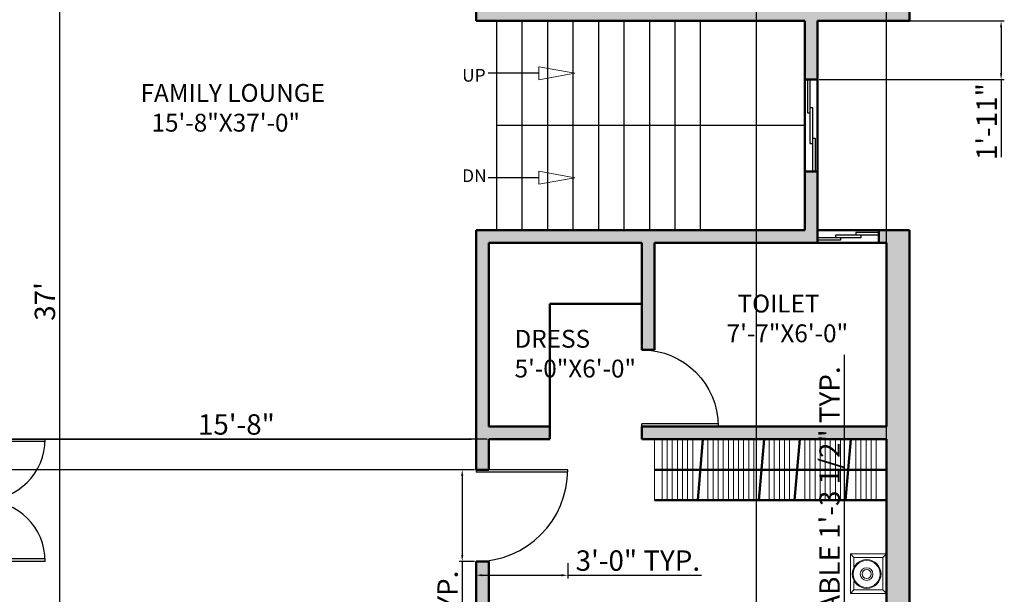
# Model space of a CAD drawing. Units: inches. Extents: x 1913 to 5309, y 1003 to 1733.
# Tile 11 of 23: x 2850 to 3237, y 1263 to 1488. Entities that reach past the tile are written whole.
import ezdxf

# ---------------------------------------------------------------- set-up
doc = ezdxf.new("R2010")
doc.units = ezdxf.units.IN
for name, color, linetype, lineweight in [('0.15', 34, 'Continuous', 15), ('A-ANNO-DIMS', 2, 'Continuous', 18), ('A-ANNO-SYMB', 1, 'Continuous', 18), ('A-ANNO-TEXT', 7, 'Continuous', 18), ('A-AREA-IDEN', 3, 'Continuous', 18), ('A-DOOR', 4, 'Continuous', 25), ('A-FLOR-PATT', 252, 'Continuous', 13), ('A-FLOR-STRS', 7, 'Continuous', 25), ('A-FURN', 8, 'Continuous', 18), ('A-GLAZ', 5, 'Continuous', 25), ('A-WALL', 7, 'Continuous', 50)]:
    doc.layers.add(name, color=color, linetype=linetype, lineweight=lineweight)
doc.styles.get("Standard").update_dxf_attribs({"font": 'arial.ttf'})
doc.dimstyles.new('ISO-25', dxfattribs={"dimtxt": 8, "dimasz": 2.5, "dimexe": 1.25, "dimexo": 0.625, "dimtad": 1, "dimdec": 1, "dimlunit": 3, "dimtxsty": 'Standard', "dimcen": 2.5, "dimclrd": 256, "dimclrt": 1, "dimadec": 0, "dimazin": 0, "dimtfac": 1, "dimtdec": 1, "dimtmove": 0, "dimatfit": 3, "dimfxl": 1, "dimarcsym": 0})

# ---------------------------------------------------------------- blocks, each defined once
blk = doc.blocks.new('VELADOR')
at = {"layer": '0.15'}
for p, q in [((-0.248, 0), (-0.203, -0.045)), ((0.248, 0), (0.202, -0.045)), ((-0.203, -0.405), (-0.248, -0.45)), ((0.248, -0.45), (0.202, -0.405))]:
    blk.add_line(p, q, dxfattribs=at)
blk.add_lwpolyline([(-0.248, 0), (-0.248, -0.45), (0.248, -0.45), (0.248, 0)], close=True, dxfattribs=at)
blk.add_lwpolyline([(0.092, -0.405), (0.202, -0.405), (0.202, -0.045), (-0.203, -0.045), (-0.203, -0.405), (-0.082, -0.405)], dxfattribs=at)
for radius in [0.18, 0.169, 0.0788, 0.0563]:
    blk.add_circle((0.005, -0.247), radius, dxfattribs=at)
blk = doc.blocks.new('*D48')
at = {"layer": 'A-ANNO-DIMS', "color": 0, "lineweight": -2, "transparency": 16777216}
for p, q in [((2859.93, 1599.96), (2867.23, 1599.96)), ((2865.98, 1597.46), (2865.98, 1158.43)), ((2859.93, 1155.93), (2867.23, 1155.93))]:
    blk.add_line(p, q, dxfattribs=at)
at = {"layer": 'A-ANNO-DIMS', "color": 0, "transparency": 16777216}
for points in [[(2865.56, 1597.46), (2866.39, 1597.46), (2865.98, 1599.96)], [(2865.56, 1158.43), (2866.39, 1158.43), (2865.98, 1155.93)]]:
    blk.add_solid(points, dxfattribs=at)
at = {"layer": 'Defpoints', "color": 0, "transparency": 16777216}
for p in [(2859.31, 1599.96), (2859.31, 1155.93), (2865.98, 1155.93)]:
    blk.add_point(p, dxfattribs=at)
at = {"layer": 'A-ANNO-DIMS', "color": 0, "transparency": 16777216, "insert": (2861.26, 1377.95), "char_height": 8, "attachment_point": 5, "rotation": 90}
blk.add_mtext("37'", dxfattribs=at)
blk = doc.blocks.new('*D49')
at = {"layer": 'A-ANNO-DIMS', "color": 0, "lineweight": -2, "transparency": 16777216}
for p, q in [((2841.34, 1324.59), (2841.34, 1325.21)), ((3029.34, 1324.59), (3029.34, 1325.21)), ((2843.84, 1323.96), (3026.84, 1323.96))]:
    blk.add_line(p, q, dxfattribs=at)
at = {"layer": 'A-ANNO-DIMS', "color": 0, "transparency": 16777216}
for points in [[(2843.84, 1324.38), (2843.84, 1323.55), (2841.34, 1323.96)], [(3026.84, 1324.38), (3026.84, 1323.55), (3029.34, 1323.96)]]:
    blk.add_solid(points, dxfattribs=at)
at = {"layer": 'Defpoints', "color": 0, "transparency": 16777216}
for p in [(2841.34, 1323.96), (3029.34, 1323.96), (3029.34, 1323.96)]:
    blk.add_point(p, dxfattribs=at)
at = {"layer": 'A-ANNO-DIMS', "color": 0, "transparency": 16777216, "insert": (2935.34, 1328.67), "char_height": 8, "attachment_point": 5}
blk.add_mtext('15\'-8"', dxfattribs=at)
blk = doc.blocks.new("MD D 4'")
for p, q in [((0, 24), (0, 0)), ((1, 24), (1, 0)), ((47, 24), (47, 0)), ((48, 24), (48, 0)), ((0, 0), (1, 0)), ((48, 0), (47, 0))]:
    blk.add_line(p, q)
for centre, start, end in [((0, 0), 0, 90), ((48, 0), 90, 180)]:
    blk.add_arc(centre, 24, start, end)
blk = doc.blocks.new("D1 3'")
for p, q in [((0, 36), (0, 0)), ((1, 36), (1, 0)), ((0, 0), (1, 0))]:
    blk.add_line(p, q)
blk.add_arc((0, 0), 36, 0, 90)
blk = doc.blocks.new("D2 2'6")
for p, q in [((0, 30), (0, 0)), ((1, 30), (1, 0)), ((0, 0), (1, 0))]:
    blk.add_line(p, q)
blk.add_arc((0, 0), 30, 0, 90)
blk = doc.blocks.new('WIN-24')
for p, q in [((0, 15), (0, 24)), ((1, 7), (1, 24)), ((2, 17), (1, 17)), ((2, 0), (2, 17)), ((1, 15), (0, 15)), ((3, 9), (2, 9)), ((3, 0), (3, 9)), ((2, 7), (1, 7))]:
    blk.add_line(p, q)
blk = doc.blocks.new('WIN-36')
for p, q in [((0, 23), (0, 36)), ((1, 11), (1, 36)), ((2, 25), (1, 25)), ((2, 0), (2, 25)), ((1, 23), (0, 23)), ((3, 13), (2, 13)), ((3, 0), (3, 13)), ((2, 11), (1, 11))]:
    blk.add_line(p, q)
blk = doc.blocks.new('*D55')
at = {"layer": 'A-ANNO-DIMS', "lineweight": -2, "transparency": 16777216}
for p, q in [((3173.87, 1195.51), (3173.87, 1356.99)), ((3173.87, 1182.46), (3173.87, 1193.01))]:
    blk.add_line(p, q, dxfattribs=at)
at = {"layer": 'A-ANNO-DIMS', "color": 0, "lineweight": -2, "transparency": 16777216}
for p, q in [((3175.58, 1195.51), (3172.62, 1195.51)), ((3175.58, 1179.96), (3172.62, 1179.96))]:
    blk.add_line(p, q, dxfattribs=at)
at = {"layer": 'A-ANNO-DIMS', "transparency": 16777216}
for points in [[(3173.45, 1193.01), (3174.29, 1193.01), (3173.87, 1195.51)], [(3173.45, 1182.46), (3174.29, 1182.46), (3173.87, 1179.96)]]:
    blk.add_solid(points, dxfattribs=at)
at = {"layer": 'Defpoints', "color": 0, "transparency": 16777216}
for p in [(3173.87, 1195.51), (3176.2, 1195.51), (3176.2, 1179.96)]:
    blk.add_point(p, dxfattribs=at)
at = {"layer": 'A-ANNO-DIMS', "color": 1, "transparency": 16777216, "insert": (3169.1, 1277.5), "char_height": 8, "attachment_point": 5, "rotation": 90}
blk.add_mtext('BEDSIDE TABLE 1\'-3 1/2" TYP.', dxfattribs=at)
blk = doc.blocks.new('*D71')
at = {"layer": 'A-ANNO-DIMS', "color": 0, "lineweight": -2, "transparency": 16777216}
for p, q in [((3028.71, 1311.96), (3022.69, 1311.96)), ((3028.71, 1275.96), (3022.69, 1275.96))]:
    blk.add_line(p, q, dxfattribs=at)
at = {"layer": 'A-ANNO-DIMS', "lineweight": -2, "transparency": 16777216}
for p, q in [((3023.94, 1309.46), (3023.94, 1278.46)), ((3023.94, 1275.96), (3023.94, 1206.46))]:
    blk.add_line(p, q, dxfattribs=at)
at = {"layer": 'A-ANNO-DIMS', "transparency": 16777216}
for points in [[(3023.52, 1309.46), (3024.36, 1309.46), (3023.94, 1311.96)], [(3023.52, 1278.46), (3024.36, 1278.46), (3023.94, 1275.96)]]:
    blk.add_solid(points, dxfattribs=at)
at = {"layer": 'Defpoints', "color": 0, "transparency": 16777216}
for p in [(3029.34, 1311.96), (3023.94, 1275.96), (3029.34, 1275.96)]:
    blk.add_point(p, dxfattribs=at)
at = {"layer": 'A-ANNO-DIMS', "color": 1, "transparency": 16777216, "insert": (3019.23, 1239.96), "char_height": 8, "attachment_point": 5, "rotation": 90}
blk.add_mtext('D1 3\'-0" TYP.', dxfattribs=at)
blk = doc.blocks.new('*D72')
at = {"layer": 'A-ANNO-DIMS', "color": 0, "lineweight": -2, "transparency": 16777216}
for p, q in [((3029.34, 1275.34), (3029.34, 1269.31)), ((3065.34, 1275.34), (3065.34, 1269.31))]:
    blk.add_line(p, q, dxfattribs=at)
at = {"layer": 'A-ANNO-DIMS', "lineweight": -2, "transparency": 16777216}
for p, q in [((3031.84, 1270.56), (3062.84, 1270.56)), ((3065.34, 1270.56), (3117.85, 1270.56))]:
    blk.add_line(p, q, dxfattribs=at)
at = {"layer": 'A-ANNO-DIMS', "transparency": 16777216}
for points in [[(3031.84, 1270.98), (3031.84, 1270.15), (3029.34, 1270.56)], [(3062.84, 1270.98), (3062.84, 1270.15), (3065.34, 1270.56)]]:
    blk.add_solid(points, dxfattribs=at)
at = {"layer": 'Defpoints', "color": 0, "transparency": 16777216}
for p in [(3029.34, 1275.96), (3065.34, 1275.96), (3065.34, 1270.56)]:
    blk.add_point(p, dxfattribs=at)
at = {"layer": 'A-ANNO-DIMS', "color": 1, "transparency": 16777216, "insert": (3092.84, 1275.28), "char_height": 8, "attachment_point": 5}
blk.add_mtext('3\'-0" TYP.', dxfattribs=at)
blk = doc.blocks.new('*D122')
at = {"layer": 'A-ANNO-DIMS', "color": 0, "lineweight": -2, "transparency": 16777216}
for p, q in [((3163.96, 1487.96), (3236.59, 1487.96)), ((3163.96, 1464.96), (3236.59, 1464.96))]:
    blk.add_line(p, q, dxfattribs=at)
at = {"layer": 'A-ANNO-DIMS', "lineweight": -2, "transparency": 16777216}
for p, q in [((3235.34, 1485.46), (3235.34, 1467.46)), ((3235.34, 1464.96), (3235.34, 1434.49))]:
    blk.add_line(p, q, dxfattribs=at)
at = {"layer": 'A-ANNO-DIMS', "transparency": 16777216}
for points in [[(3234.92, 1485.46), (3235.76, 1485.46), (3235.34, 1487.96)], [(3234.92, 1467.46), (3235.76, 1467.46), (3235.34, 1464.96)]]:
    blk.add_solid(points, dxfattribs=at)
at = {"layer": 'Defpoints', "color": 0, "transparency": 16777216}
for p in [(3163.34, 1487.96), (3163.34, 1464.96), (3235.34, 1464.96)]:
    blk.add_point(p, dxfattribs=at)
at = {"layer": 'A-ANNO-DIMS', "color": 1, "transparency": 16777216, "insert": (3230.7, 1448.47), "char_height": 8, "attachment_point": 5, "rotation": 90}
blk.add_mtext('1\'-11"', dxfattribs=at)
blk = doc.blocks.new('*D126')
at = {"layer": 'A-ANNO-DIMS', "color": 0, "lineweight": -2, "transparency": 16777216}
for p, q in [((3139.34, 1180.59), (3139.34, 1724.21)), ((3190.34, 1180.59), (3190.34, 1724.21))]:
    blk.add_line(p, q, dxfattribs=at)
at = {"layer": 'A-ANNO-DIMS', "lineweight": -2, "transparency": 16777216}
blk.add_line((3141.84, 1722.96), (3187.84, 1722.96), dxfattribs=at)
at = {"layer": 'A-ANNO-DIMS', "transparency": 16777216}
for points in [[(3141.84, 1723.38), (3141.84, 1722.55), (3139.34, 1722.96)], [(3187.84, 1723.38), (3187.84, 1722.55), (3190.34, 1722.96)]]:
    blk.add_solid(points, dxfattribs=at)
at = {"layer": 'Defpoints', "color": 0, "transparency": 16777216}
for p in [(3190.34, 1722.96), (3139.34, 1179.96), (3190.34, 1179.96)]:
    blk.add_point(p, dxfattribs=at)
at = {"layer": 'A-ANNO-DIMS', "color": 1, "transparency": 16777216, "insert": (3164.84, 1727.68), "char_height": 8, "attachment_point": 5}
blk.add_mtext('4\'-3"', dxfattribs=at)
blk = doc.blocks.new('*D127')
at = {"layer": 'A-ANNO-DIMS', "lineweight": -2, "transparency": 16777216}
for p, q in [((2611.34, 1323.96), (2611.34, 1348.23)), ((2611.34, 1314.46), (2611.34, 1321.46))]:
    blk.add_line(p, q, dxfattribs=at)
at = {"layer": 'A-ANNO-DIMS', "color": 0, "lineweight": -2, "transparency": 16777216}
for p, q in [((3033.71, 1323.96), (2610.09, 1323.96)), ((3028.71, 1311.96), (2610.09, 1311.96))]:
    blk.add_line(p, q, dxfattribs=at)
at = {"layer": 'A-ANNO-DIMS', "transparency": 16777216}
for points in [[(2610.92, 1321.46), (2611.76, 1321.46), (2611.34, 1323.96)], [(2610.92, 1314.46), (2611.76, 1314.46), (2611.34, 1311.96)]]:
    blk.add_solid(points, dxfattribs=at)
at = {"layer": 'Defpoints', "color": 0, "transparency": 16777216}
for p in [(2611.34, 1323.96), (3034.34, 1323.96), (3029.34, 1311.96)]:
    blk.add_point(p, dxfattribs=at)
at = {"layer": 'A-ANNO-DIMS', "color": 1, "transparency": 16777216, "insert": (2606.63, 1337.35), "char_height": 8, "attachment_point": 5, "rotation": 90}
blk.add_mtext('1\'-0"', dxfattribs=at)

msp = doc.modelspace()

# ---------------------------------------------------------------- hatches: boundary and pattern name
at = {"layer": 'A-FLOR-PATT'}
h = msp.add_hatch(color=256, dxfattribs=at)
h.dxf.hatch_style = 1
h.paths.add_polyline_path([(2841.34, 1686.96), (2683.34, 1686.96), (2683.34, 1625.96), (2692.34, 1625.96), (2692.34, 1677.96), (2836.34, 1677.96), (2836.34, 1554.96), (2841.34, 1554.96), (2841.34, 1599.96), (2859.31, 1599.96), (2859.31, 1608.96), (2841.34, 1608.96)])
h.paths.add_polyline_path([(3034.34, 1625.46), (3029.34, 1625.46), (3029.34, 1608.96), (2955.31, 1608.96), (2955.31, 1599.96), (3029.34, 1599.96), (3029.34, 1528.96), (3034.34, 1528.96)])
h.paths.add_polyline_path([(3199.34, 1686.96), (3029.34, 1686.96), (3029.34, 1661.46), (3034.34, 1661.46), (3034.34, 1677.96), (3190.34, 1677.96), (3190.34, 1492.96), (3029.34, 1492.96), (3029.34, 1487.96), (3158.34, 1487.96), (3158.34, 1464.96), (3163.34, 1464.96), (3163.34, 1487.96), (3199.34, 1487.96)])
h.paths.add_polyline_path([(3099.34, 1400.96), (3163.34, 1400.96), (3163.34, 1428.96), (3158.34, 1428.96), (3158.34, 1405.96), (3029.34, 1405.96), (3029.34, 1311.96), (3034.34, 1311.96), (3034.34, 1323.96), (3058.34, 1323.96), (3058.34, 1328.96), (3034.34, 1328.96), (3034.34, 1400.96), (3094.34, 1400.96), (3094.34, 1358.96), (3099.34, 1358.96)])
h.paths.add_polyline_path([(3199.34, 1405.96), (3187.34, 1405.96), (3187.34, 1400.96), (3190.34, 1400.96), (3190.34, 1328.96), (3094.34, 1328.96), (3094.34, 1323.96), (3190.34, 1323.96), (3190.34, 1299.96), (3190.34, 1179.96), (3176.2, 1179.96), (3139.34, 1179.96), (3139.34, 1170.96), (3190.34, 1170.96), (3190.34, 1146.96), (3199.34, 1146.96)])
h.paths.add_polyline_path([(3085.34, 1179.96), (3064.34, 1179.96), (3064.34, 1170.96), (3085.34, 1170.96)])
h.paths.add_polyline_path([(3029.34, 1158.98), (3029.34, 1199.59, 0.414216), (3026.32, 1202.59), (3010.47, 1202.59, 0.414214), (3007.47, 1199.59), (3007.47, 1181.52, 0.46174), (3009.2, 1180.04), (3026.11, 1180.04, 0.414263), (3025.52, 1179.45), (3025.52, 1162.57, 0.41435), (3026.11, 1161.97), (3007.38, 1161.97, 0.41842), (3006.78, 1161.36, 0.785879), (3005.87, 1162.09, 0.298637), (3006.77, 1163.46), (3006.77, 1178.53, 0.414214), (3005.27, 1180.02), (2990.22, 1180.02, 0.416116), (2988.72, 1178.51, 0.414208), (2987.21, 1180.02), (2987.2, 1180.02, -0.413869), (2988.7, 1178.52, -0.412492), (2990.21, 1180.02), (2990.21, 1180.03), (3005.27, 1180.02, -0.414213), (3006.77, 1178.53, -0.414214), (3008.27, 1180.02), (3008.14, 1180.27, -0.252555), (3007.47, 1181.52), (3007.45, 1181.51), (3007.47, 1199.59, -0.414214), (3010.47, 1202.59), (3026.33, 1202.59, -0.414214), (3029.34, 1199.59), (3029.34, 1275.96), (3034.34, 1275.96), (3034.34, 1146.96), (3011.34, 1146.96), (3011.34, 1155.96), (2951.06, 1155.96, -0.414214), (2948.06, 1158.97), (2948.06, 1158.97, 0.421637), (2951.14, 1155.96), (3026.4, 1155.96, 0.407251)])
h.paths.add_polyline_path([(2845.34, 1275.96), (2836.34, 1275.96), (2836.34, 1233.96), (2845.34, 1233.96), (2845.34, 1237.71)])
h.paths.add_polyline_path([(2845.34, 1173.96), (2836.34, 1173.96), (2836.34, 1146.96), (2863.34, 1146.96), (2863.34, 1155.93), (2848.48, 1155.93, -0.414214), (2845.34, 1159.07)])
h.paths.add_polyline_path([(2841.34, 1356.96), (2836.34, 1356.96), (2836.34, 1328.96), (2793.34, 1328.96), (2793.34, 1405.96), (2841.34, 1405.96), (2841.34, 1470.96), (2836.34, 1470.96), (2836.34, 1410.96), (2769.34, 1410.96), (2769.34, 1513.96), (2836.34, 1513.96), (2836.34, 1506.96), (2841.34, 1506.96), (2841.34, 1518.96), (2764.34, 1518.96), (2764.34, 1405.96), (2788.34, 1405.96), (2788.34, 1328.96), (2692.34, 1328.96), (2692.34, 1340.96), (2683.34, 1340.96), (2683.34, 1323.96), (2841.34, 1323.96)])
h.paths.add_polyline_path([(2692.34, 1513.96), (2734.34, 1513.96), (2734.34, 1518.96), (2692.34, 1518.96), (2692.34, 1571.96), (2683.34, 1571.96), (2683.34, 1420.96), (2683.34, 1364.96), (2692.34, 1364.96), (2692.34, 1405.96), (2734.34, 1405.96), (2734.34, 1410.96), (2692.34, 1410.96)])

# ---------------------------------------------------------------- linework, layer by layer
at = {"layer": 'A-ANNO-SYMB'}
for points in [[(3068.16, 1467.46), (3054, 1470.02), (3054, 1464.91)], [(3068.16, 1426.46), (3054, 1423.91), (3054, 1429.02)]]:
    msp.add_lwpolyline(points, close=True, dxfattribs=at)
at = {"layer": 'A-FLOR-STRS'}
for p, q in [((3037.34, 1487.96), (3037.34, 1405.96)), ((3047.34, 1487.96), (3047.34, 1405.96)), ((3057.34, 1487.96), (3057.34, 1405.96)), ((3067.34, 1487.96), (3067.34, 1405.96)), ((3077.34, 1487.96), (3077.34, 1405.96)), ((3087.34, 1487.96), (3087.34, 1405.96)), ((3097.34, 1487.96), (3097.34, 1405.96)), ((3107.34, 1487.96), (3107.34, 1405.96)), ((3117.34, 1487.96), (3117.34, 1405.96)), ((3054, 1467.46), (3034.08, 1467.46)), ((3158.34, 1446.96), (3037.34, 1446.96)), ((3054, 1426.46), (3034.08, 1426.46))]:
    msp.add_line(p, q, dxfattribs=at)
at = {"layer": 'A-FURN'}
for p, q in [((3099.34, 1323.96), (3099.34, 1299.96)), ((3102.34, 1323.96), (3102.34, 1299.96)), ((3104.34, 1323.96), (3104.34, 1299.96)), ((3106.34, 1323.96), (3106.34, 1299.96)), ((3108.34, 1323.96), (3108.34, 1299.96)), ((3110.34, 1323.96), (3110.34, 1299.96)), ((3112.34, 1323.96), (3112.34, 1299.96)), ((3114.34, 1323.96), (3114.34, 1299.96)), ((3120.34, 1323.96), (3120.34, 1299.96)), ((3122.34, 1323.96), (3122.34, 1299.96)), ((3124.34, 1323.96), (3124.34, 1299.96)), ((3126.34, 1323.96), (3126.34, 1299.96)), ((3128.34, 1323.96), (3128.34, 1299.96)), ((3128.34, 1323.96), (3128.34, 1299.96)), ((3130.34, 1323.96), (3130.34, 1299.96)), ((3132.34, 1323.96), (3132.34, 1299.96)), ((3134.34, 1323.96), (3134.34, 1299.96)), ((3136.34, 1323.96), (3136.34, 1299.96)), ((3138.34, 1323.96), (3138.34, 1299.96)), ((3144.34, 1323.96), (3144.34, 1299.96)), ((3146.34, 1323.96), (3146.34, 1299.96)), ((3148.34, 1323.96), (3148.34, 1299.96)), ((3150.34, 1323.96), (3150.34, 1299.96)), ((3152.34, 1323.96), (3152.34, 1299.96)), ((3158.34, 1323.96), (3158.34, 1299.96)), ((3160.34, 1323.96), (3160.34, 1299.96)), ((3162.34, 1323.96), (3162.34, 1299.96)), ((3164.34, 1323.96), (3164.34, 1299.96)), ((3166.34, 1323.96), (3166.34, 1299.96)), ((3168.34, 1323.96), (3168.34, 1299.96)), ((3170.34, 1323.96), (3170.34, 1299.96)), ((3172.34, 1323.96), (3172.34, 1299.96)), ((3178.34, 1323.96), (3178.34, 1299.96)), ((3180.34, 1323.96), (3180.34, 1299.96)), ((3182.34, 1323.96), (3182.34, 1299.96)), ((3184.34, 1323.96), (3184.34, 1299.96)), ((3186.34, 1323.96), (3186.34, 1299.96)), ((3190.34, 1323.96), (3190.34, 1299.96))]:
    msp.add_line(p, q, dxfattribs=at)
at = {"layer": 'A-WALL'}
for p, q in [((3199.34, 1686.96), (3199.34, 1487.96)), ((3029.34, 1492.96), (3029.34, 1487.96)), ((3029.34, 1487.96), (3158.34, 1487.96)), ((3158.34, 1487.96), (3158.34, 1405.96)), ((3163.34, 1487.96), (3199.34, 1487.96)), ((3163.34, 1487.96), (3163.34, 1400.96)), ((3163.34, 1464.96), (3158.34, 1464.96)), ((3163.34, 1428.96), (3158.34, 1428.96)), ((3029.34, 1405.96), (3158.34, 1405.96)), ((3029.34, 1405.96), (3029.34, 1311.96)), ((3163.34, 1405.96), (3199.34, 1405.96)), ((3187.34, 1405.96), (3187.34, 1400.96)), ((3199.34, 1405.96), (3199.34, 1098.96)), ((3034.34, 1400.96), (3094.34, 1400.96)), ((3034.34, 1400.96), (3034.34, 1328.96)), ((3094.34, 1400.96), (3094.34, 1358.96)), ((3099.34, 1400.96), (3190.34, 1400.96)), ((3099.34, 1400.96), (3099.34, 1358.96)), ((3190.34, 1400.96), (3190.34, 1328.96)), ((3058.34, 1376.96), (3094.34, 1376.96)), ((3058.34, 1376.96), (3058.34, 1323.96)), ((3094.34, 1358.96), (3099.34, 1358.96)), ((3034.34, 1328.96), (3058.34, 1328.96)), ((3094.34, 1328.96), (3190.34, 1328.96)), ((3094.34, 1328.96), (3094.34, 1323.96)), ((3034.34, 1323.96), (3058.34, 1323.96)), ((3034.34, 1323.96), (3034.34, 1311.96)), ((3094.34, 1323.96), (3190.34, 1323.96)), ((3118.34, 1323.96), (3116.34, 1299.96)), ((3142.34, 1323.96), (3140.34, 1299.96)), ((3156.34, 1323.96), (3154.34, 1299.96)), ((3176.34, 1323.96), (3174.34, 1299.96)), ((3190.34, 1323.96), (3190.34, 1179.96)), ((3029.34, 1311.96), (3034.34, 1311.96)), ((3190.34, 1311.96), (3099.34, 1311.96)), ((3099.34, 1299.96), (3190.34, 1299.96)), ((3029.34, 1275.96), (3034.34, 1275.96)), ((3029.34, 1275.96), (3029.34, 1155.96)), ((3034.34, 1275.96), (3034.34, 1146.96))]:
    msp.add_line(p, q, dxfattribs=at)

# ---------------------------------------------------------------- block references
at = {"layer": 'A-DOOR', "xscale": -1, "rotation": 270}
msp.add_blockref("D2 2'6", (3094.34, 1328.96), dxfattribs=at)
at = {"layer": 'A-DOOR', "rotation": 270}
for name, p in [("MD D 4'", (2836.34, 1323.96)), ("D1 3'", (3029.34, 1311.96))]:
    msp.add_blockref(name, p, dxfattribs=at)
at = {"layer": 'A-FURN', "xscale": 31.41542173157097, "yscale": 31.41542173157097, "zscale": 31.41542173157097, "rotation": 270}
msp.add_blockref('VELADOR', (3190.34, 1271.19), dxfattribs=at)
at = {"layer": 'A-GLAZ'}
for name, p, rotation in [('WIN-36', (3162.34, 1464.96), 180), ('WIN-24', (3187.34, 1401.96), 89.99999999999156)]:
    msp.add_blockref(name, p, dxfattribs=dict(at, rotation=rotation))

# ---------------------------------------------------------------- texts
at = {"layer": 'A-ANNO-TEXT', "char_height": 5}
for s, insert, attachment_point in [('{UP}', (3023.9, 1469.16), 1), ('{DN}', (3023.9, 1424.77), 7)]:
    msp.add_mtext_dynamic_manual_height_columns(s, width=10.7355, gutter_width=12.5, heights=[0], dxfattribs=dict(at, insert=insert, attachment_point=attachment_point))
at = {"layer": 'A-AREA-IDEN', "char_height": 7, "attachment_point": 1}
for s, insert in [('FAMILY LOUNGE\\P  15\'-8"X37\'-0"', (2897.76, 1463.24)), ('  TOILET\\P7\'-7"X6\'-0"', (3127.65, 1380.62)), ('DRESS\\P5\'-0"X6\'-0"', (3044.45, 1366.8))]:
    msp.add_mtext_dynamic_manual_height_columns(s, width=86.9528, gutter_width=12.5, heights=[0], dxfattribs=dict(at, insert=insert))

# ---------------------------------------------------------------- dimensions: what is measured, and where the dimension line sits
at = {"layer": 'A-ANNO-DIMS'}
for base, p1, p2, override, picture, middle in [((3190.34, 1722.96), (3139.34, 1179.96), (3190.34, 1179.96), {"dimdec": 1, "dimlfac": 1, "dimrnd": 0, "dimzin": 1, "dimdsep": 46, "dimlunit": 4, "dimfrac": 2}, '*D126', (3164.84, 1727.68)), ((3029.34, 1323.96), (2841.34, 1323.96), (3029.34, 1323.96), {"dimclrd": 0, "dimclre": 0, "dimclrt": 0}, '*D49', (2935.34, 1328.67))]:
    dim = msp.add_linear_dim(base=base, p1=p1, p2=p2, dimstyle='ISO-25', override=override, dxfattribs=at)
    dim.commit()
    dim.dimension.update_dxf_attribs({"geometry": picture, "text_midpoint": middle})
for base, p1, p2, override, picture, middle in [((2865.98, 1155.93), (2859.31, 1599.96), (2859.31, 1155.93), {"dimclrd": 0, "dimclre": 0, "dimclrt": 0}, '*D48', (2861.26, 1377.95)), ((3235.34, 1464.96), (3163.34, 1487.96), (3163.34, 1464.96), {"dimdec": 1, "dimlfac": 1, "dimrnd": 0, "dimzin": 1, "dimdsep": 46, "dimlunit": 4, "dimfrac": 2}, '*D122', (3230.7, 1448.47)), ((2611.34, 1323.96), (3029.34, 1311.96), (3034.34, 1323.96), {"dimdec": 1, "dimlfac": 1, "dimrnd": 0, "dimzin": 1, "dimdsep": 46, "dimlunit": 4, "dimfrac": 2}, '*D127', (2606.63, 1337.35))]:
    dim = msp.add_linear_dim(base=base, p1=p1, p2=p2, angle=90, dimstyle='ISO-25', override=override, dxfattribs=at)
    dim.commit()
    dim.dimension.update_dxf_attribs({"geometry": picture, "text_midpoint": middle})
for base, p1, p2, angle, text, picture, middle in [((3173.869, 1195.5147), (3176.2016, 1179.9641), (3176.2016, 1195.5147), 90, 'BEDSIDE TABLE <> TYP.', '*D55', (3169.1049, 1277.5046)), ((3023.94, 1275.96), (3029.34, 1311.96), (3029.34, 1275.96), 270, 'D1 <> TYP.', '*D71', (3019.23, 1239.96))]:
    dim = msp.add_linear_dim(base=base, p1=p1, p2=p2, angle=angle, text=text, dimstyle='ISO-25', override={"dimdec": 1, "dimrnd": 0, "dimzin": 1, "dimlunit": 4, "dimfrac": 2}, dxfattribs=at)
    dim.commit()
    dim.dimension.update_dxf_attribs({"geometry": picture, "text_midpoint": middle})
dim = msp.add_linear_dim(base=(3065.34, 1270.56), p1=(3029.34, 1275.96), p2=(3065.34, 1275.96), text='<> TYP.', dimstyle='ISO-25', override={"dimdec": 1, "dimrnd": 0, "dimzin": 1, "dimlunit": 4, "dimfrac": 2}, dxfattribs=at)
dim.commit()
dim.dimension.update_dxf_attribs({"geometry": '*D72', "text_midpoint": (3092.84, 1275.28)})

doc.saveas('drawing.dxf')
